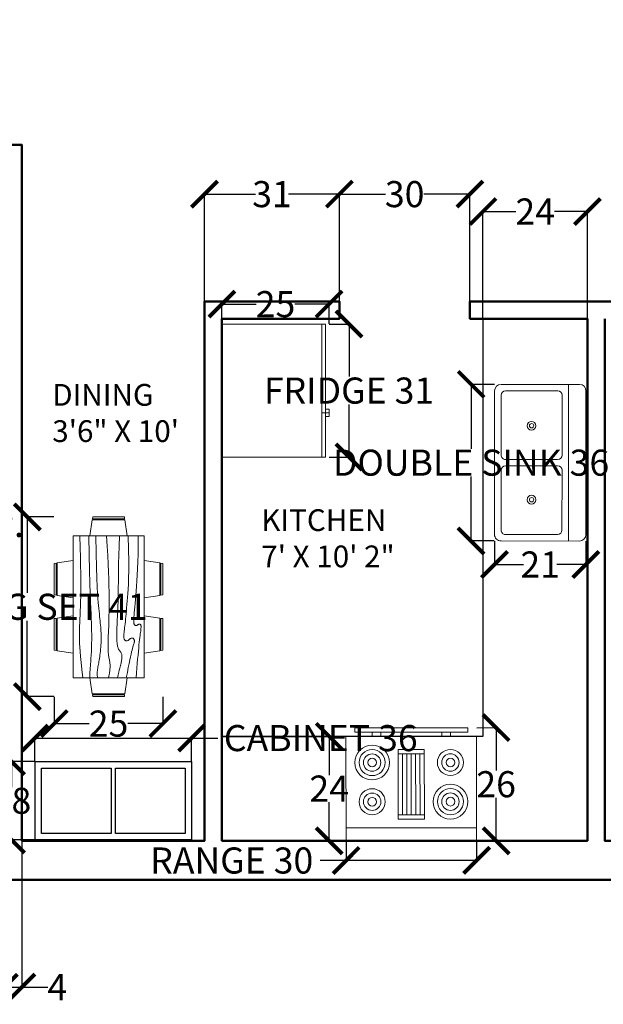
# Model space of a CAD drawing. Units: inches. Extents: x 9 to 573, y -373 to 44.
# Tile 2 of 5: x 195 to 329, y -373 to -146. Entities that reach past the tile are written whole.
import ezdxf

# ---------------------------------------------------------------- set-up
doc = ezdxf.new("R2010")
doc.units = ezdxf.units.IN
doc.header["$MEASUREMENT"] = 0
for name, color, linetype, lineweight in [('A-ANNO-DIMS', 2, 'Continuous', 18), ('A-AREA-IDEN', 7, 'Continuous', 25), ('A-EQPM', 8, 'Continuous', 18), ('A-FLOR-CASE', 8, 'Continuous', 25), ('A-FLOR-FIXT', 9, 'Continuous', 18), ('A-FURN', 8, 'Continuous', 18), ('A-WALL', 7, 'Continuous', 50)]:
    doc.layers.add(name, color=color, linetype=linetype, lineweight=lineweight)
doc.styles.get("Standard").update_dxf_attribs({"font": 'arial.ttf'})
doc.dimstyles.get("Standard").update_dxf_attribs({"dimtxt": 6, "dimasz": 6, "dimexe": 0.18, "dimexo": 0.0625, "dimgap": 0.09, "dimtad": 0, "dimtih": 1, "dimtoh": 1, "dimdec": 0, "dimzin": 0, "dimdsep": 46, "dimlunit": 4, "dimtxsty": 'Standard', "dimblk": 'ARCHTICK', "dimcen": 0.09, "dimadec": 0, "dimazin": 0, "dimtfac": 1, "dimtdec": 0, "dimtofl": 0, "dimtmove": 0, "dimatfit": 3, "dimldrblk": 'ARCHTICK', "dimfxl": 1, "dimtolj": 1, "dimtzin": 0, "dimarcsym": 0})

# ---------------------------------------------------------------- blocks, each defined once
blk = doc.blocks.new('Dining Set - 36 x 72 in.')
for p, q in [((-22.2343, 26.00059), (-23.4847, 17.99762)), ((-22.2304, 26), (-5.7608, 26)), ((-22, 27.5), (-22.1562, 26.50042)), ((-5.8416, 26.5), (-22.1534, 26.5)), ((-22, 27.5), (-6, 27.5)), ((-5.8437, 26.49966), (-6, 27.5)), ((-4.5152, 17.99762), (-5.7655, 25.99926)), ((5.7657, 26.00059), (4.5153, 17.99762)), ((5.7696, 26), (22.2392, 26)), ((6, 27.5), (5.8438, 26.50042)), ((22.1584, 26.5), (5.8466, 26.5)), ((6, 27.5), (22, 27.5)), ((22.1563, 26.49966), (22, 27.5)), ((23.4848, 17.99762), (22.2345, 25.99926)), ((36, 18), (-36, 18)), ((-36, 18), (-36, -18)), ((36, -18), (36, 18)), ((-45.5, 8), (-44.5004, 8.15617)), ((-45.5, 8), (-45.5, -8)), ((-44.5, -8.15843), (-44.5, 8.15338)), ((-44.0006, 8.23428), (-35.9976, 9.48474)), ((-44, 8.23041), (-44, -8.23915)), ((44.0006, 8.23428), (35.9976, 9.48474)), ((44, 8.23041), (44, -8.23915)), ((44.5, -8.15843), (44.5, 8.15338)), ((45.5, 8), (44.5005, 8.15617)), ((45.5, 8), (45.5, -8)), ((-44.4997, -8.15631), (-45.5, -8)), ((-35.9976, -9.48476), (-43.9993, -8.2345)), ((35.9976, -9.48476), (43.9993, -8.2345)), ((44.4997, -8.15631), (45.5, -8)), ((-36, -18), (36, -18)), ((-22.2343, -26.0006), (-23.4847, -17.99762)), ((-4.5152, -17.99762), (-5.7655, -25.99928)), ((5.7657, -26.0006), (4.5153, -17.99762)), ((23.4848, -17.99762), (22.2345, -25.99928)), ((-22.2304, -26), (-5.7608, -26)), ((-22, -27.5), (-22.1562, -26.50044)), ((-5.8416, -26.5), (-22.1534, -26.5)), ((-22, -27.5), (-6, -27.5)), ((-5.8437, -26.49967), (-6, -27.5)), ((5.7696, -26), (22.2392, -26)), ((6, -27.5), (5.8438, -26.50044)), ((22.1584, -26.5), (5.8466, -26.5)), ((6, -27.5), (22, -27.5)), ((22.1563, -26.49967), (22, -27.5))]:
    blk.add_line(p, q)
for points in [[(-36, 15), (-31.1772, 14.97754), (-26.8079, 14.91406), (-22.8538, 14.81543), (-19.276, 14.6875), (-16.0362, 14.53613), (-13.0957, 14.36718), (-10.4159, 14.18652), (-7.9583, 14), (-5.6904, 13.81315), (-3.6035, 13.63021), (-1.6954, 13.45508), (0.0365, 13.29166), (1.5945, 13.14388), (2.9811, 13.01562), (4.1988, 12.9108), (5.25, 12.83333), (6.1393, 12.78613), (6.8802, 12.76823), (7.4883, 12.77767), (7.9792, 12.8125), (8.3685, 12.87077), (8.6719, 12.95052), (8.9049, 13.0498), (9.0833, 13.16666), (9.2205, 13.29899), (9.3216, 13.44401), (9.3895, 13.59879), (9.4271, 13.76041), (9.4373, 13.92594), (9.4232, 14.09245), (9.3875, 14.257), (9.3333, 14.41666), (9.2638, 14.56917), (9.1836, 14.71484), (9.0975, 14.85465), (9.0104, 14.98958), (8.9272, 15.1206), (8.8529, 15.2487), (8.7922, 15.37483), (8.75, 15.5), (8.7305, 15.62467), (8.7344, 15.74739), (8.7617, 15.86621), (8.8125, 15.97916), (8.8867, 16.08431), (8.9844, 16.17968), (9.1055, 16.26334), (9.25, 16.33333), (9.4189, 16.38802), (9.6172, 16.42708), (9.8506, 16.45052), (10.125, 16.45833), (10.4463, 16.45052), (10.8203, 16.42708), (11.2529, 16.38802), (11.75, 16.33333), (12.3184, 16.26318), (12.9694, 16.17838), (13.7151, 16.07991), (14.5677, 15.96875), (15.5395, 15.84586), (16.6426, 15.71224), (17.8893, 15.56884), (19.2917, 15.41666), (20.859, 15.25667), (22.5879, 15.08984), (24.4721, 14.91715), (26.5052, 14.73958), (28.6809, 14.5581), (30.9929, 14.3737), (33.4347, 14.18733), (36, 14)], [(-36, 10), (-28.9766, 10.14274), (-23.1725, 10.20442), (-18.4241, 10.19775), (-14.5677, 10.13541), (-11.4399, 10.03011), (-8.877, 9.89453), (-6.7154, 9.74137), (-4.7917, 9.58333), (-2.9698, 9.43082), (-1.2246, 9.28515), (0.4415, 9.14534), (2.026, 9.01041), (3.5266, 8.87939), (4.9408, 8.7513), (6.266, 8.62516), (7.5, 8.5), (8.6411, 8.37549), (9.6914, 8.2539), (10.6538, 8.13818), (11.5312, 8.03125), (12.3267, 7.93603), (13.043, 7.85547), (13.6831, 7.79248), (14.25, 7.75), (14.7471, 7.7303), (15.1797, 7.73307), (15.5537, 7.75732), (15.875, 7.80208), (16.1494, 7.86637), (16.3828, 7.94922), (16.5811, 8.04964), (16.75, 8.16666), (16.8944, 8.29915), (17.0143, 8.44531), (17.1089, 8.60319), (17.1771, 8.77083), (17.218, 8.94629), (17.2305, 9.1276), (17.2137, 9.31282), (17.1667, 9.5), (17.0895, 9.6875), (16.987, 9.875), (16.8649, 10.0625), (16.7292, 10.25), (16.5856, 10.4375), (16.4401, 10.625), (16.2985, 10.8125), (16.1667, 11), (16.05, 11.18733), (15.9518, 11.3737), (15.8752, 11.5581), (15.8229, 11.73958), (15.798, 11.91715), (15.8034, 12.08984), (15.842, 12.25667), (15.9167, 12.41666), (16.0295, 12.56836), (16.1784, 12.70833), (16.3605, 12.83268), (16.5729, 12.9375), (16.8127, 13.01888), (17.0768, 13.07291), (17.3625, 13.0957), (17.6667, 13.08333), (17.9894, 13.03312), (18.3418, 12.94726), (18.7382, 12.82918), (19.1927, 12.68229), (19.7195, 12.51001), (20.3327, 12.31575), (21.0465, 12.10294), (21.875, 11.875), (22.8357, 11.63354), (23.959, 11.37304), (25.2786, 11.08618), (26.8282, 10.76562), (28.6414, 10.40405), (30.752, 9.99414), (33.1936, 9.52856), (36, 9)], [(-36, 5.5), (-30.7157, 5.3348), (-26.069, 5.20963), (-21.9946, 5.11767), (-18.4271, 5.05208), (-15.3009, 5.00602), (-12.5508, 4.97265), (-10.1112, 4.94515), (-7.9167, 4.91666), (-5.909, 4.88167), (-4.0586, 4.83984), (-2.3429, 4.79215), (-0.7396, 4.73958), (0.7739, 4.6831), (2.22, 4.6237), (3.6213, 4.56233), (5, 4.5), (6.373, 4.43782), (7.7344, 4.3776), (9.0723, 4.32129), (10.375, 4.27083), (11.6309, 4.22819), (12.8281, 4.19531), (13.9551, 4.17415), (15, 4.16666), (15.954, 4.17448), (16.819, 4.19791), (17.6001, 4.23698), (18.3021, 4.29166), (18.9299, 4.36198), (19.4883, 4.44791), (19.9823, 4.54948), (20.4167, 4.66666), (20.7969, 4.79899), (21.1302, 4.94401), (21.4245, 5.09879), (21.6875, 5.26041), (21.9271, 5.42594), (22.1511, 5.59245), (22.3672, 5.757), (22.5834, 5.91666), (22.8065, 6.06868), (23.0404, 6.21093), (23.2879, 6.34147), (23.5521, 6.45833), (23.8358, 6.55957), (24.142, 6.64323), (24.4735, 6.70735), (24.8334, 6.75), (25.2235, 6.76969), (25.642, 6.76692), (26.0858, 6.74267), (26.5521, 6.69791), (27.0379, 6.63362), (27.5404, 6.55078), (28.0565, 6.45036), (28.5834, 6.33333), (29.1242, 6.19987), (29.7071, 6.04687), (30.3661, 5.87044), (31.1354, 5.66666), (32.0493, 5.43164), (33.142, 5.16146), (34.4475, 4.85221), (36, 4.5)], [(-36, -1), (-30.7915, -0.6591), (-26.0195, -0.38216), (-21.6519, -0.16284), (-17.6563, 0.00521), (-14.0005, 0.12833), (-10.6523, 0.21289), (-7.5796, 0.26522), (-4.75, 0.29166), (-2.134, 0.29793), (0.2878, 0.28711), (2.5317, 0.26163), (4.6146, 0.22396), (6.5529, 0.17651), (8.3633, 0.12174), (10.0623, 0.06209), (11.6667, 0), (13.1899, -0.06201), (14.6341, -0.1211), (15.9982, -0.17432), (17.2813, -0.21875), (18.4823, -0.25147), (19.6003, -0.26953), (20.6343, -0.27002), (21.5834, -0.25), (22.4481, -0.20768), (23.2357, -0.14584), (23.9549, -0.06836), (24.6146, 0.02083), (25.2235, 0.11784), (25.7904, 0.21875), (26.3241, 0.31966), (26.8334, 0.41666), (27.3265, 0.50618), (27.8099, 0.58593), (28.2894, 0.65397), (28.7709, 0.70833), (29.2601, 0.74707), (29.763, 0.76823), (30.2855, 0.76985), (30.8334, 0.75), (31.4088, 0.70784), (31.9994, 0.64713), (32.589, 0.57275), (33.1615, 0.48958), (33.7008, 0.4025), (34.1908, 0.3164), (34.6153, 0.23616), (34.9584, 0.16666), (35.2099, 0.11165), (35.3848, 0.07031), (35.504, 0.04069), (35.5886, 0.02083), (35.6594, 0.00879), (35.7377, 0.0026), (35.8442, 0.00032), (36, 0)], [(-36, -6.5), (-27.1843, -6.31267), (-20.084, -6.1263), (-14.469, -5.9419), (-10.1094, -5.76042), (-6.7752, -5.58285), (-4.2363, -5.41016), (-2.2629, -5.24333), (-0.625, -5.08334), (0.8708, -4.93099), (2.2715, -4.78646), (3.5872, -4.64974), (4.8281, -4.52084), (6.0046, -4.39974), (7.127, -4.28646), (8.2053, -4.18099), (9.25, -4.08334), (10.2705, -3.99382), (11.2734, -3.91407), (12.2647, -3.84603), (13.25, -3.79167), (14.2354, -3.75293), (15.2266, -3.73177), (16.2295, -3.73015), (17.25, -3.75), (18.2912, -3.79248), (19.3451, -3.85547), (20.4009, -3.93604), (21.4479, -4.03125), (22.4754, -4.13819), (23.4727, -4.25391), (24.4289, -4.37549), (25.3334, -4.5), (26.1785, -4.62492), (26.9694, -4.74935), (27.7145, -4.87281), (28.4219, -4.99479), (29.1, -5.11483), (29.7572, -5.23242), (30.4016, -5.34709), (31.0417, -5.45834), (31.6837, -5.56437), (32.3262, -5.65821), (32.9658, -5.73153), (33.599, -5.77604), (34.2224, -5.78345), (34.8327, -5.74545), (35.4264, -5.65373), (36, -5.5)], [(-36, -10), (-26.4022, -9.81299), (-18.4675, -9.62891), (-11.9839, -9.45069), (-6.7396, -9.28125), (-2.5226, -9.12354), (0.8789, -8.98047), (3.6769, -8.85498), (6.0833, -8.75), (8.2767, -8.66765), (10.3021, -8.60677), (12.1712, -8.56543), (13.8958, -8.54167), (15.4876, -8.53353), (16.9583, -8.53907), (18.3197, -8.55632), (19.5834, -8.58334), (20.7616, -8.61841), (21.8685, -8.66081), (22.9188, -8.71004), (23.9271, -8.76563), (24.9081, -8.82707), (25.8763, -8.89388), (26.8465, -8.96558), (27.8334, -9.04167), (28.8474, -9.12118), (29.8828, -9.20117), (30.93, -9.27824), (31.9792, -9.34896), (33.0205, -9.40991), (34.0443, -9.45768), (35.0407, -9.48885), (36, -9.5)], [(-36, -14.5), (-30.0881, -14.33513), (-25.0332, -14.21224), (-20.7312, -14.12647), (-17.0781, -14.07292), (-13.97, -14.04671), (-11.3027, -14.04297), (-8.9724, -14.05681), (-6.875, -14.08334), (-4.9224, -14.11833), (-3.0905, -14.16016), (-1.3709, -14.20785), (0.2448, -14.26042), (1.7647, -14.3169), (3.1973, -14.3763), (4.5507, -14.43767), (5.8333, -14.5), (7.0554, -14.5621), (8.235, -14.62175), (9.3922, -14.67652), (10.5469, -14.72396), (11.7192, -14.76164), (12.929, -14.78711), (14.1965, -14.79794), (15.5417, -14.79167), (16.9933, -14.76424), (18.6152, -14.70508), (20.4804, -14.60197), (22.6615, -14.44271), (25.2312, -14.21509), (28.2624, -13.9069), (31.8277, -13.50594), (36, -13)]]:
    blk.add_lwpolyline(points)
blk = doc.blocks.new('Range-Oven - 30 in top')
for p, q in [((0, -3), (30, -3)), ((12, -6), (18, -6)), ((13, -20), (13, -6)), ((14, -6), (14, -20)), ((15, -20), (15, -6)), ((16, -6), (16, -20)), ((17, -20), (17, -6)), ((18, -20), (12, -20)), ((6, -24), (6, -25)), ((8, -25), (8, -24)), ((22, -25), (22, -24)), ((24, -24), (24, -25))]:
    blk.add_line(p, q)
for points in [[(0, -24), (0, 0), (30, 0), (30, -24)], [(12, -21), (12, -5), (18, -5), (18, -21)], [(2, -26), (2, -25), (28, -25), (28, -26)]]:
    blk.add_lwpolyline(points, close=True)
for centre, radius in [((6, -9), 4), ((6, -9), 3), ((24, -9), 3), ((6, -9), 2), ((6, -9), 1), ((24, -9), 2), ((24, -9), 1), ((6, -18), 3), ((24, -18), 4), ((24, -18), 3), ((6, -18), 2), ((6, -18), 1), ((24, -18), 2), ((24, -18), 1)]:
    blk.add_circle(centre, radius)
blk = doc.blocks.new('Sink-double - 36 in top')
for p, q in [((-18, -4), (18, -4)), ((-0.75, -18.5), (-0.75, -6.5)), ((0.75, -6.5), (0.75, -18.5))]:
    blk.add_line(p, q)
for points in [[(-16.5, 0), (16.5, 0)], [(-18, -19.5), (-18, -1.5)], [(18, -1.5), (18, -19.5)], [(-16.5, -18.5), (-16.5, -6.5)], [(-15.5, -5.5), (-1.75, -5.5)], [(1.75, -5.5), (15.5, -5.5)], [(16.5, -6.5), (16.5, -18.5)], [(-1.75, -19.5), (-15.5, -19.5)], [(15.5, -19.5), (1.75, -19.5)], [(16.5, -21), (-16.5, -21)]]:
    blk.add_lwpolyline(points)
for centre, radius in [((-8.5, -12.5), 1), ((-8.5, -12.5), 0.5), ((8.5, -12.5), 1), ((8.5, -12.5), 0.5)]:
    blk.add_circle(centre, radius)
for centre, radius, start, end in [((-16.5, -1.5), 1.5, 90, 180), ((16.5, -1.5), 1.5, 0, 90), ((-15.5, -6.5), 1, 90, 180), ((-1.75, -6.5), 1, 0, 90), ((1.75, -6.5), 1, 90, 180), ((15.5, -6.5), 1, 0, 90), ((-16.5, -19.5), 1.5, 180, 270), ((-15.5, -18.5), 1, 180, 270), ((-1.75, -18.5), 1, 270, 0), ((1.75, -18.5), 1, 180, 270), ((15.5, -18.5), 1, 270, 0), ((16.5, -19.5), 1.5, 270, 0)]:
    blk.add_arc(centre, radius, start, end)
blk = doc.blocks.new('Refrigerator-2 door - 36 in top')
for p, q in [((0, -26.999999), (36, -26.999999)), ((11, -27.999999), (11, -28.999999)), ((11, -28.999999), (13, -28.999999)), ((12, -26.999999), (12, -28.999999)), ((13, -28.999999), (13, -27.999999))]:
    blk.add_line(p, q)
blk.add_lwpolyline([(0, -27.999999), (0, 0), (36, 0), (36, -27.999999)], close=True)
blk = doc.blocks.new('Wall Cabinet - 18 x 36 in front')
for p, q in [((17.5, -1.5), (17.5, -16.5)), ((18.5, -16.5), (18.5, -1.5))]:
    blk.add_line(p, q)
blk.add_lwpolyline([(0, -18), (0, 0), (36, 0), (36, -18)], close=True)
for points in [[(17.5, -16.5), (1.5, -16.5), (1.5, -1.5), (17.5, -1.5)], [(18.5, -1.5), (34.5, -1.5), (34.5, -16.5), (18.5, -16.5)]]:
    blk.add_lwpolyline(points)
blk = doc.blocks.new('_ArchTick')
at = {"color": 0, "linetype": 'ByBlock', "const_width": 0.15}
blk.add_lwpolyline([(-0.5, -0.5), (0.5, 0.5)], dxfattribs=at)
blk = doc.blocks.new('*D39')
at = {"layer": 'A-ANNO-DIMS', "color": 0, "lineweight": -2, "transparency": 16777216}
for p, q in [((141.31, -262.66), (161.44, -262.44)), ((141.35, -266.28), (141.31, -262.48)), ((161.48, -266.06), (161.44, -262.26)), ((161.44, -262.44), (167.44, -262.37))]:
    blk.add_line(p, q, dxfattribs=at)
at = {"layer": 'Defpoints', "color": 0, "transparency": 16777216}
for p in [(161.44, -262.44), (141.35, -266.35), (161.49, -266.12)]:
    blk.add_point(p, dxfattribs=at)
at = {"layer": 'A-ANNO-DIMS', "color": 0, "lineweight": -2, "transparency": 16777216, "xscale": 6, "yscale": 6, "zscale": 6}
for p, rotation in [((141.31, -262.66), 180.6375101586001), ((161.44, -262.44), 0.6375101586001275)]:
    blk.add_blockref('_ArchTick', p, dxfattribs=dict(at, rotation=rotation))
at = {"layer": 'A-ANNO-DIMS', "color": 0, "transparency": 16777216, "insert": (182.19, -262.37), "char_height": 6, "attachment_point": 5}
blk.add_mtext('\\A1;20 TYP.', dxfattribs=at)
blk = doc.blocks.new('*D46')
at = {"layer": 'A-ANNO-DIMS', "color": 0, "lineweight": -2, "transparency": 16777216}
for p, q in [((202.92, -260.76), (196.6, -260.76)), ((196.78, -260.76), (196.78, -278.22)), ((196.78, -302.06), (196.78, -284.61)), ((202.92, -302.06), (196.6, -302.06))]:
    blk.add_line(p, q, dxfattribs=at)
at = {"layer": 'Defpoints', "color": 0, "transparency": 16777216}
for p in [(202.98, -260.76), (196.78, -302.06), (202.98, -302.06)]:
    blk.add_point(p, dxfattribs=at)
at = {"layer": 'A-ANNO-DIMS', "color": 0, "lineweight": -2, "transparency": 16777216, "xscale": 6, "yscale": 6, "zscale": 6}
for p, rotation in [((196.78, -260.76), 90), ((196.78, -302.06), 270)]:
    blk.add_blockref('_ArchTick', p, dxfattribs=dict(at, rotation=rotation))
at = {"layer": 'A-ANNO-DIMS', "color": 0, "transparency": 16777216, "insert": (196.78, -281.41), "char_height": 6, "attachment_point": 5}
blk.add_mtext('\\A1;DINING SET 41', dxfattribs=at)
blk = doc.blocks.new('*D47')
at = {"layer": 'A-ANNO-DIMS', "color": 0, "lineweight": -2, "transparency": 16777216}
for p, q in [((202.98, -302.13), (202.98, -308.44)), ((227.94, -302.13), (227.94, -308.44)), ((202.98, -308.26), (211, -308.26)), ((227.94, -308.26), (219.92, -308.26))]:
    blk.add_line(p, q, dxfattribs=at)
at = {"layer": 'Defpoints', "color": 0, "transparency": 16777216}
for p in [(202.98, -302.06), (227.94, -302.06), (227.94, -308.26)]:
    blk.add_point(p, dxfattribs=at)
at = {"layer": 'A-ANNO-DIMS', "color": 0, "lineweight": -2, "transparency": 16777216, "xscale": 6, "yscale": 6, "zscale": 6, "rotation": 180}
blk.add_blockref('_ArchTick', (202.98, -308.26), dxfattribs=at)
at = {"layer": 'A-ANNO-DIMS', "color": 0, "lineweight": -2, "transparency": 16777216, "xscale": 6, "yscale": 6, "zscale": 6}
blk.add_blockref('_ArchTick', (227.94, -308.26), dxfattribs=at)
at = {"layer": 'A-ANNO-DIMS', "color": 0, "transparency": 16777216, "insert": (215.46, -308.26), "char_height": 6, "attachment_point": 5}
blk.add_mtext('\\A1;25', dxfattribs=at)
blk = doc.blocks.new('*D50')
at = {"layer": 'A-ANNO-DIMS', "color": 0, "lineweight": -2, "transparency": 16777216}
for p, q in [((270.05, -335.28), (270.06, -339.9)), ((300.05, -335.26), (300.06, -339.88)), ((270.06, -339.72), (264.06, -339.73)), ((300.06, -339.7), (270.06, -339.72))]:
    blk.add_line(p, q, dxfattribs=at)
at = {"layer": 'Defpoints', "color": 0, "transparency": 16777216}
for p in [(270.05, -335.22), (300.05, -335.2), (270.06, -339.72)]:
    blk.add_point(p, dxfattribs=at)
at = {"layer": 'A-ANNO-DIMS', "color": 0, "lineweight": -2, "transparency": 16777216, "xscale": 6, "yscale": 6, "zscale": 6}
for p, rotation in [((270.06, -339.72), 180.0486562224878), ((300.06, -339.7), 0.048656222487784)]:
    blk.add_blockref('_ArchTick', p, dxfattribs=dict(at, rotation=rotation))
at = {"layer": 'A-ANNO-DIMS', "color": 0, "transparency": 16777216, "insert": (243.77, -339.73), "char_height": 6, "attachment_point": 5}
blk.add_mtext('\\A1;RANGE 30', dxfattribs=at)
blk = doc.blocks.new('*D51')
at = {"layer": 'A-ANNO-DIMS', "color": 0, "lineweight": -2, "transparency": 16777216}
for p, q in [((300.09, -309.2), (304.71, -309.19)), ((304.53, -309.19), (304.54, -319.04)), ((304.55, -335.19), (304.55, -325.35)), ((300.12, -335.2), (304.73, -335.19))]:
    blk.add_line(p, q, dxfattribs=at)
at = {"layer": 'Defpoints', "color": 0, "transparency": 16777216}
for p in [(300.03, -309.2), (300.05, -335.2), (304.55, -335.19)]:
    blk.add_point(p, dxfattribs=at)
at = {"layer": 'A-ANNO-DIMS', "color": 0, "lineweight": -2, "transparency": 16777216, "xscale": 6, "yscale": 6, "zscale": 6}
for p, rotation in [((304.53, -309.19), 90.04865622248779), ((304.55, -335.19), 270.0486562224878)]:
    blk.add_blockref('_ArchTick', p, dxfattribs=dict(at, rotation=rotation))
at = {"layer": 'A-ANNO-DIMS', "color": 0, "transparency": 16777216, "insert": (304.54, -322.19), "char_height": 6, "attachment_point": 5}
blk.add_mtext('\\A1;26', dxfattribs=at)
blk = doc.blocks.new('*D52')
at = {"layer": 'A-ANNO-DIMS', "color": 0, "lineweight": -2, "transparency": 16777216}
for p, q in [((304.13, -230.28), (298.62, -230.28)), ((298.8, -230.28), (298.79, -245.08)), ((298.77, -266.28), (298.78, -251.48)), ((304.11, -266.28), (298.59, -266.28))]:
    blk.add_line(p, q, dxfattribs=at)
at = {"layer": 'Defpoints', "color": 0, "transparency": 16777216}
for p in [(304.2, -230.28), (298.77, -266.28), (304.17, -266.28)]:
    blk.add_point(p, dxfattribs=at)
at = {"layer": 'A-ANNO-DIMS', "color": 0, "lineweight": -2, "transparency": 16777216, "xscale": 6, "yscale": 6, "zscale": 6}
for p, rotation in [((298.8, -230.28), 89.96776293761982), ((298.77, -266.28), 269.9677629376198)]:
    blk.add_blockref('_ArchTick', p, dxfattribs=dict(at, rotation=rotation))
at = {"layer": 'A-ANNO-DIMS', "color": 0, "transparency": 16777216, "insert": (298.78, -248.28), "char_height": 6, "attachment_point": 5}
blk.add_mtext('\\A1;DOUBLE SINK 36', dxfattribs=at)
blk = doc.blocks.new('*D53')
at = {"layer": 'A-ANNO-DIMS', "color": 0, "lineweight": -2, "transparency": 16777216}
for p, q in [((304.17, -266.34), (304.17, -271.86)), ((325.17, -266.36), (325.17, -271.87)), ((304.17, -271.68), (310.81, -271.69)), ((325.17, -271.69), (318.53, -271.69))]:
    blk.add_line(p, q, dxfattribs=at)
at = {"layer": 'Defpoints', "color": 0, "transparency": 16777216}
for p in [(304.17, -266.28), (325.17, -266.29), (325.17, -271.69)]:
    blk.add_point(p, dxfattribs=at)
at = {"layer": 'A-ANNO-DIMS', "color": 0, "lineweight": -2, "transparency": 16777216, "xscale": 6, "yscale": 6, "zscale": 6}
for p, rotation in [((304.17, -271.68), 179.9677629376198), ((325.17, -271.69), 359.9677629376198)]:
    blk.add_blockref('_ArchTick', p, dxfattribs=dict(at, rotation=rotation))
at = {"layer": 'A-ANNO-DIMS', "color": 0, "transparency": 16777216, "insert": (314.67, -271.69), "char_height": 6, "attachment_point": 5}
blk.add_mtext('\\A1;21', dxfattribs=at)
blk = doc.blocks.new('*D54')
at = {"layer": 'A-ANNO-DIMS', "color": 0, "lineweight": -2, "transparency": 16777216}
for p, q in [((266.2, -216.42), (270.91, -216.42)), ((270.73, -216.42), (270.73, -228.51)), ((270.73, -246.99), (270.73, -234.9)), ((266.2, -246.99), (270.91, -246.99))]:
    blk.add_line(p, q, dxfattribs=at)
at = {"layer": 'Defpoints', "color": 0, "transparency": 16777216}
for p in [(266.14, -216.42), (270.73, -216.42), (266.14, -246.99)]:
    blk.add_point(p, dxfattribs=at)
at = {"layer": 'A-ANNO-DIMS', "color": 0, "lineweight": -2, "transparency": 16777216, "xscale": 6, "yscale": 6, "zscale": 6}
for p, rotation in [((270.73, -216.42), 90), ((270.73, -246.99), 270)]:
    blk.add_blockref('_ArchTick', p, dxfattribs=dict(at, rotation=rotation))
at = {"layer": 'A-ANNO-DIMS', "color": 0, "transparency": 16777216, "insert": (270.73, -231.71), "char_height": 6, "attachment_point": 5}
blk.add_mtext('\\A1;FRIDGE 31', dxfattribs=at)
blk = doc.blocks.new('*D55')
at = {"layer": 'A-ANNO-DIMS', "color": 0, "lineweight": -2, "transparency": 16777216}
for p, q in [((241.52, -216.36), (241.52, -211.66)), ((241.52, -211.84), (249.37, -211.84)), ((266.14, -211.84), (258.29, -211.84)), ((266.14, -216.36), (266.14, -211.66))]:
    blk.add_line(p, q, dxfattribs=at)
at = {"layer": 'Defpoints', "color": 0, "transparency": 16777216}
for p in [(241.52, -211.84), (241.52, -216.42), (266.14, -216.42)]:
    blk.add_point(p, dxfattribs=at)
at = {"layer": 'A-ANNO-DIMS', "color": 0, "lineweight": -2, "transparency": 16777216, "xscale": 6, "yscale": 6, "zscale": 6, "rotation": 180}
blk.add_blockref('_ArchTick', (241.52, -211.84), dxfattribs=at)
at = {"layer": 'A-ANNO-DIMS', "color": 0, "lineweight": -2, "transparency": 16777216, "xscale": 6, "yscale": 6, "zscale": 6}
blk.add_blockref('_ArchTick', (266.14, -211.84), dxfattribs=at)
at = {"layer": 'A-ANNO-DIMS', "color": 0, "transparency": 16777216, "insert": (253.83, -211.84), "char_height": 6, "attachment_point": 5}
blk.add_mtext('\\A1;25', dxfattribs=at)
blk = doc.blocks.new('*D56')
at = {"layer": 'A-ANNO-DIMS', "color": 0, "lineweight": -2, "transparency": 16777216}
for p, q in [((198.55, -316.93), (198.55, -311.41)), ((198.55, -311.59), (234.55, -311.59)), ((234.55, -316.93), (234.55, -311.41)), ((234.55, -311.59), (240.55, -311.59))]:
    blk.add_line(p, q, dxfattribs=at)
at = {"layer": 'Defpoints', "color": 0, "transparency": 16777216}
for p in [(234.55, -311.59), (198.55, -316.99), (234.55, -316.99)]:
    blk.add_point(p, dxfattribs=at)
at = {"layer": 'A-ANNO-DIMS', "color": 0, "lineweight": -2, "transparency": 16777216, "xscale": 6, "yscale": 6, "zscale": 6, "rotation": 180}
blk.add_blockref('_ArchTick', (198.55, -311.59), dxfattribs=at)
at = {"layer": 'A-ANNO-DIMS', "color": 0, "lineweight": -2, "transparency": 16777216, "xscale": 6, "yscale": 6, "zscale": 6}
blk.add_blockref('_ArchTick', (234.55, -311.59), dxfattribs=at)
at = {"layer": 'A-ANNO-DIMS', "color": 0, "transparency": 16777216, "insert": (264.23, -311.59), "char_height": 6, "attachment_point": 5}
blk.add_mtext('\\A1;CABINET 36', dxfattribs=at)
blk = doc.blocks.new('*D57')
at = {"layer": 'A-ANNO-DIMS', "color": 0, "lineweight": -2, "transparency": 16777216}
for p, q in [((198.49, -316.99), (192.97, -316.99)), ((193.15, -316.99), (193.15, -322.84)), ((193.15, -334.99), (193.15, -329.14)), ((198.49, -334.99), (192.97, -334.99))]:
    blk.add_line(p, q, dxfattribs=at)
at = {"layer": 'Defpoints', "color": 0, "transparency": 16777216}
for p in [(193.15, -316.99), (198.55, -316.99), (198.55, -334.99)]:
    blk.add_point(p, dxfattribs=at)
at = {"layer": 'A-ANNO-DIMS', "color": 0, "lineweight": -2, "transparency": 16777216, "xscale": 6, "yscale": 6, "zscale": 6}
for p, rotation in [((193.15, -316.99), 90), ((193.15, -334.99), 270)]:
    blk.add_blockref('_ArchTick', p, dxfattribs=dict(at, rotation=rotation))
at = {"layer": 'A-ANNO-DIMS', "color": 0, "transparency": 16777216, "insert": (193.15, -325.99), "char_height": 6, "attachment_point": 5}
blk.add_mtext('\\A1;18', dxfattribs=at)
blk = doc.blocks.new('*D61')
at = {"layer": 'A-ANNO-DIMS', "color": 0, "lineweight": -2, "transparency": 16777216}
for p, q in [((191.52, -335.26), (191.52, -369.03)), ((195.52, -335.26), (195.52, -369.03)), ((191.52, -368.85), (195.52, -368.85)), ((195.52, -368.85), (201.52, -368.85))]:
    blk.add_line(p, q, dxfattribs=at)
at = {"layer": 'Defpoints', "color": 0, "transparency": 16777216}
for p in [(191.52, -335.2), (195.52, -335.2), (195.52, -368.85)]:
    blk.add_point(p, dxfattribs=at)
at = {"layer": 'A-ANNO-DIMS', "color": 0, "lineweight": -2, "transparency": 16777216, "xscale": 6, "yscale": 6, "zscale": 6, "rotation": 180}
blk.add_blockref('_ArchTick', (191.52, -368.85), dxfattribs=at)
at = {"layer": 'A-ANNO-DIMS', "color": 0, "lineweight": -2, "transparency": 16777216, "xscale": 6, "yscale": 6, "zscale": 6}
blk.add_blockref('_ArchTick', (195.52, -368.85), dxfattribs=at)
at = {"layer": 'A-ANNO-DIMS', "color": 0, "transparency": 16777216, "insert": (203.68, -368.85), "char_height": 6, "attachment_point": 5}
blk.add_mtext('\\A1;4', dxfattribs=at)
blk = doc.blocks.new('*D74')
at = {"layer": 'A-ANNO-DIMS', "color": 0, "lineweight": -2, "transparency": 16777216}
for p, q in [((268.52, -211.13), (268.52, -186.37)), ((268.52, -186.55), (279.14, -186.55)), ((298.52, -186.55), (287.89, -186.55)), ((298.52, -211.13), (298.52, -186.37))]:
    blk.add_line(p, q, dxfattribs=at)
at = {"layer": 'Defpoints', "color": 0, "transparency": 16777216}
for p in [(298.52, -186.55), (268.52, -211.2), (298.52, -211.2)]:
    blk.add_point(p, dxfattribs=at)
at = {"layer": 'A-ANNO-DIMS', "color": 0, "lineweight": -2, "transparency": 16777216, "xscale": 6, "yscale": 6, "zscale": 6, "rotation": 180}
blk.add_blockref('_ArchTick', (268.52, -186.55), dxfattribs=at)
at = {"layer": 'A-ANNO-DIMS', "color": 0, "lineweight": -2, "transparency": 16777216, "xscale": 6, "yscale": 6, "zscale": 6}
blk.add_blockref('_ArchTick', (298.52, -186.55), dxfattribs=at)
at = {"layer": 'A-ANNO-DIMS', "color": 0, "transparency": 16777216, "insert": (283.52, -186.55), "char_height": 6, "attachment_point": 5}
blk.add_mtext('\\A1;30', dxfattribs=at)
blk = doc.blocks.new('*D75')
at = {"layer": 'A-ANNO-DIMS', "color": 0, "lineweight": -2, "transparency": 16777216}
for p, q in [((237.52, -211.13), (237.52, -186.37)), ((237.52, -186.55), (249.21, -186.55)), ((268.52, -186.55), (256.82, -186.55)), ((268.52, -211.13), (268.52, -186.37))]:
    blk.add_line(p, q, dxfattribs=at)
at = {"layer": 'Defpoints', "color": 0, "transparency": 16777216}
for p in [(268.52, -186.55), (237.52, -211.2), (268.52, -211.2)]:
    blk.add_point(p, dxfattribs=at)
at = {"layer": 'A-ANNO-DIMS', "color": 0, "lineweight": -2, "transparency": 16777216, "xscale": 6, "yscale": 6, "zscale": 6, "rotation": 180}
blk.add_blockref('_ArchTick', (237.52, -186.55), dxfattribs=at)
at = {"layer": 'A-ANNO-DIMS', "color": 0, "lineweight": -2, "transparency": 16777216, "xscale": 6, "yscale": 6, "zscale": 6}
blk.add_blockref('_ArchTick', (268.52, -186.55), dxfattribs=at)
at = {"layer": 'A-ANNO-DIMS', "color": 0, "transparency": 16777216, "insert": (253.02, -186.55), "char_height": 6, "attachment_point": 5}
blk.add_mtext('\\A1;31', dxfattribs=at)
blk = doc.blocks.new('*D93')
at = {"layer": 'A-ANNO-DIMS', "color": 0, "lineweight": -2, "transparency": 16777216}
for p, q in [((241.58, -311.2), (266.35, -311.2)), ((266.17, -311.2), (266.17, -320.09)), ((266.17, -335.2), (266.17, -326.3)), ((241.58, -335.2), (266.35, -335.2))]:
    blk.add_line(p, q, dxfattribs=at)
at = {"layer": 'Defpoints', "color": 0, "transparency": 16777216}
for p in [(241.52, -311.2), (241.52, -335.2), (266.17, -335.2)]:
    blk.add_point(p, dxfattribs=at)
at = {"layer": 'A-ANNO-DIMS', "color": 0, "lineweight": -2, "transparency": 16777216, "xscale": 6, "yscale": 6, "zscale": 6}
for p, rotation in [((266.17, -311.2), 90), ((266.17, -335.2), 270)]:
    blk.add_blockref('_ArchTick', p, dxfattribs=dict(at, rotation=rotation))
at = {"layer": 'A-ANNO-DIMS', "color": 0, "transparency": 16777216, "insert": (266.17, -323.2), "char_height": 6, "attachment_point": 5}
blk.add_mtext('\\A1;24', dxfattribs=at)
blk = doc.blocks.new('*D94')
at = {"layer": 'A-ANNO-DIMS', "color": 0, "lineweight": -2, "transparency": 16777216}
for p, q in [((301.52, -215.13), (301.52, -190.37)), ((301.52, -190.55), (309.09, -190.55)), ((325.52, -190.55), (317.94, -190.55)), ((325.52, -215.13), (325.52, -190.37))]:
    blk.add_line(p, q, dxfattribs=at)
at = {"layer": 'Defpoints', "color": 0, "transparency": 16777216}
for p in [(325.52, -190.55), (301.52, -215.2), (325.52, -215.2)]:
    blk.add_point(p, dxfattribs=at)
at = {"layer": 'A-ANNO-DIMS', "color": 0, "lineweight": -2, "transparency": 16777216, "xscale": 6, "yscale": 6, "zscale": 6, "rotation": 180}
blk.add_blockref('_ArchTick', (301.52, -190.55), dxfattribs=at)
at = {"layer": 'A-ANNO-DIMS', "color": 0, "lineweight": -2, "transparency": 16777216, "xscale": 6, "yscale": 6, "zscale": 6}
blk.add_blockref('_ArchTick', (325.52, -190.55), dxfattribs=at)
at = {"layer": 'A-ANNO-DIMS', "color": 0, "transparency": 16777216, "insert": (313.52, -190.55), "char_height": 6, "attachment_point": 5}
blk.add_mtext('\\A1;24', dxfattribs=at)

msp = doc.modelspace()

# ---------------------------------------------------------------- linework, layer by layer
at = {"layer": 'A-FLOR-CASE'}
msp.add_lwpolyline([(301.5169, -215.1966), (301.5169, -311.1966), (241.5169, -311.1966)], dxfattribs=at)
at = {"layer": 'A-WALL'}
for p, q in [((195.5169, -215.1966), (195.5169, -211.1966)), ((325.5169, -215.1966), (325.5169, -335.1966))]:
    msp.add_line(p, q, dxfattribs=at)
for points in [[(329.5169, -215.1966), (329.5169, -335.1966), (509.5169, -335.1966), (518.5169, -335.1966), (518.5169, -344.1966), (38.5169, -344.1966), (38.5169, 15.8034), (518.5169, 15.8034), (518.5169, -117.1966), (450.7536, -117.1966), (450.7536, -140.1966), (446.7536, -140.1966), (446.7536, -117.1966), (431.5169, -117.1966), (431.5169, -113.1966), (509.5169, -113.1966), (509.5169, 6.8034), (389.5169, 6.8034), (389.5169, -113.1966), (395.5169, -113.1966), (395.5169, -117.1966), (385.5169, -117.1966), (385.5169, 6.8034), (325.5169, 6.8034)], [(195.5169, -211.1966), (195.5169, -175.1966), (186.5169, -175.1966)], [(450.7536, -211.1966), (450.7536, -188.1966), (446.7536, -188.1966), (446.7536, -211.1966), (298.5169, -211.1966), (298.5169, -215.1966), (325.5169, -215.1966), (325.5169, -335.1966), (241.5169, -335.1966), (241.5169, -215.1966), (268.5169, -215.1966), (268.5169, -211.1966), (241.5169, -211.1966), (237.5169, -211.1966), (237.5169, -215.1966), (237.5169, -335.1966), (195.5169, -335.1966), (195.5169, -215.1966)]]:
    msp.add_lwpolyline(points, dxfattribs=at)

# ---------------------------------------------------------------- block references
at = {"layer": 'A-EQPM', "xscale": 0.8491152459887572, "yscale": 0.8491152459887572, "zscale": 0.8491152459887572, "rotation": 90}
msp.add_blockref('Refrigerator-2 door - 36 in top', (241.5169, -246.9915), dxfattribs=at)
at = {"layer": 'A-EQPM', "rotation": 180.0486562224878}
msp.add_blockref('Range-Oven - 30 in top', (300.0545, -335.1966), dxfattribs=at)
at = {"layer": 'A-FLOR-CASE'}
msp.add_blockref('Wall Cabinet - 18 x 36 in front', (198.5545, -316.9915), dxfattribs=at)
at = {"layer": 'A-FLOR-FIXT', "rotation": 269.9677629376198}
msp.add_blockref('Sink-double - 36 in top', (325.185, -248.2935), dxfattribs=at)
at = {"layer": 'A-FURN', "xscale": 0.4538727027399741, "yscale": 0.4538727027399741, "zscale": 0.4538727027399741, "rotation": 270}
msp.add_blockref('Dining Set - 36 x 72 in.', (215.4601, -281.4133), dxfattribs=at)

# ---------------------------------------------------------------- texts
at = {"layer": 'A-AREA-IDEN', "char_height": 5, "attachment_point": 1}
for s, width, insert in [('DINING \\P3\'6" X 10\'', 37.537595, (202.5169, -230.1966)), ('KITCHEN \\P7\' X 10\' 2"', 74.962405, (250.5545, -258.9915))]:
    msp.add_mtext_dynamic_manual_height_columns(s, width=width, gutter_width=1, heights=[0], dxfattribs=dict(at, insert=insert))

# ---------------------------------------------------------------- dimensions: what is measured, and where the dimension line sits
at = {"layer": 'A-ANNO-DIMS'}
for base, p1, p2, picture, middle in [((268.5169, -186.5466), (237.5169, -211.1966), (268.5169, -211.1966), '*D75', (253.0169, -186.5466)), ((325.5169, -190.5466), (301.5169, -215.1966), (325.5169, -215.1966), '*D94', (313.5169, -190.5466)), ((227.9416, -308.2599), (202.9786, -302.0645), (227.9416, -302.0645), '*D47', (215.4601, -308.2599)), ((195.5169, -368.8466), (191.5169, -335.1966), (195.5169, -335.1966), '*D61', (203.6819, -368.8466))]:
    dim = msp.add_linear_dim(base=base, p1=p1, p2=p2, dimstyle='Standard', override={"dimdec": 0, "dimlfac": 1, "dimrnd": 0, "dimzin": 0, "dimdsep": 46, "dimlunit": 2}, dxfattribs=at)
    dim.commit()
    dim.dimension.update_dxf_attribs({"geometry": picture, "text_midpoint": middle})
for base, p1, p2, angle, picture, middle in [((298.5169, -186.5466), (268.5169, -211.1966), (298.5169, -211.1966), 0, '*D74', (283.5169, -186.5466)), ((241.5169, -211.8381), (266.1412, -216.4233), (241.5169, -216.4233), 180, '*D55', (253.829, -211.8381)), ((325.1718, -271.6935), (304.1749, -266.2817), (325.1749, -266.2935), 359.967763, '*D53', (314.6718, -271.6876)), ((304.5545, -335.1928), (300.0324, -309.1966), (300.0545, -335.1966), 270.048656, '*D51', (304.5434, -322.1928)), ((266.1669, -335.1966), (241.5169, -311.1966), (241.5169, -335.1966), 270, '*D93', (266.1669, -323.1966)), ((193.1545, -316.9915), (198.5545, -334.9915), (198.5545, -316.9915), 90, '*D57', (193.1545, -325.9915))]:
    dim = msp.add_linear_dim(base=base, p1=p1, p2=p2, angle=angle, dimstyle='Standard', override={"dimdec": 0, "dimlfac": 1, "dimrnd": 0, "dimzin": 0, "dimdsep": 46, "dimlunit": 2}, dxfattribs=at)
    dim.commit()
    dim.dimension.update_dxf_attribs({"geometry": picture, "text_midpoint": middle})
for base, p1, p2, angle, text, picture, middle in [((270.7264, -216.4233), (266.1412, -246.9915), (266.1412, -216.4233), 90, 'FRIDGE <>', '*D54', (270.7264, -231.7074)), ((298.7749, -266.2786), (304.1951, -230.2817), (304.1749, -266.2817), 269.967763, 'DOUBLE SINK <>', '*D52', (298.785, -248.2786)), ((161.4447, -262.4391), (141.3503, -266.3455), (161.4856, -266.1215), 0.63751, '<> TYP.', '*D39', (182.1885, -262.3723)), ((196.7832, -302.0645), (202.9786, -260.7621), (202.9786, -302.0645), 270, 'DINING SET <>', '*D46', (196.7832, -281.4133)), ((270.0583, -339.7221), (300.0545, -335.1966), (270.0545, -335.2221), 180.048656, 'RANGE <>', '*D50', (243.7684, -339.7272))]:
    dim = msp.add_linear_dim(base=base, p1=p1, p2=p2, angle=angle, text=text, dimstyle='Standard', override={"dimdec": 0, "dimlfac": 1, "dimrnd": 0, "dimzin": 0, "dimdsep": 46, "dimlunit": 2}, dxfattribs=at)
    dim.commit()
    dim.dimension.update_dxf_attribs({"geometry": picture, "text_midpoint": middle})
dim = msp.add_linear_dim(base=(234.5545, -311.5915), p1=(198.5545, -316.9915), p2=(234.5545, -316.9915), text='CABINET <>', dimstyle='Standard', override={"dimdec": 0, "dimlfac": 1, "dimrnd": 0, "dimzin": 0, "dimdsep": 46, "dimlunit": 2}, dxfattribs=at)
dim.commit()
dim.dimension.update_dxf_attribs({"geometry": '*D56', "text_midpoint": (264.2331, -311.5915)})

doc.saveas('drawing.dxf')
